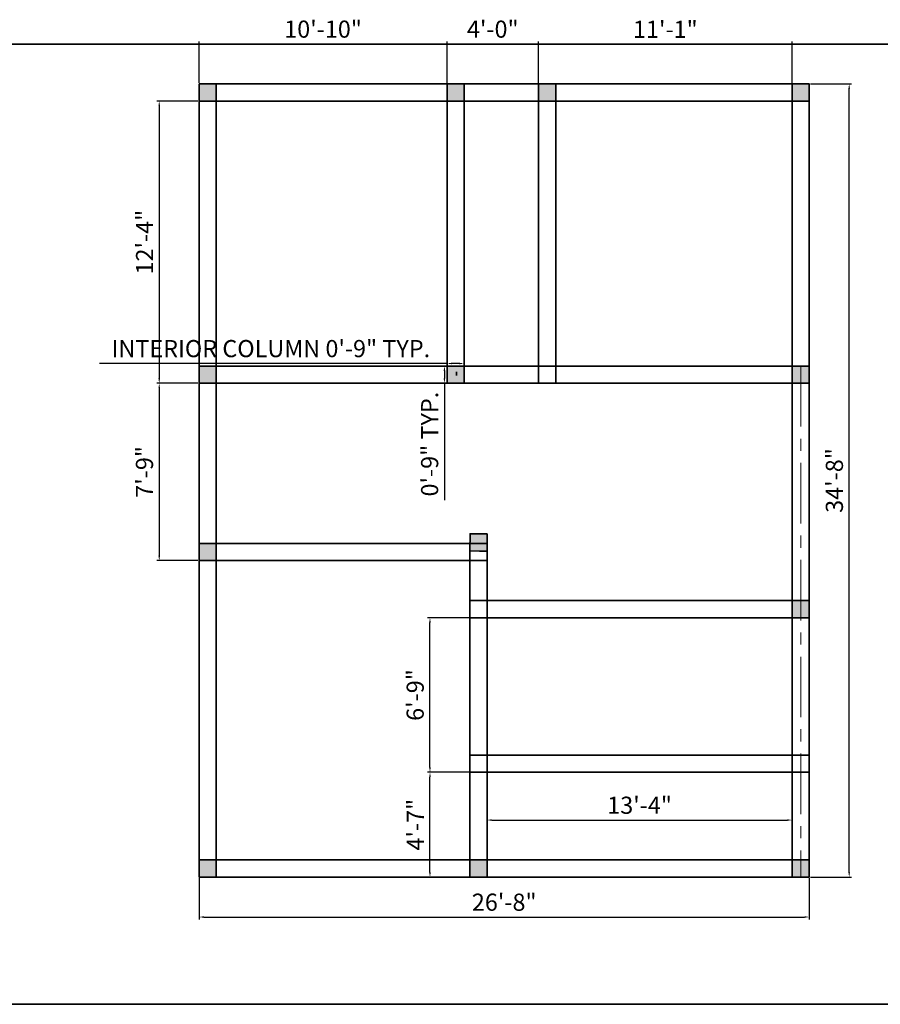
# Model space of a CAD drawing. Units: inches. Extents: x 2289 to 3796, y 1741 to 2286.
# Tile 3 of 4: x 2741 to 3192, y 1742 to 2258. Entities that reach past the tile are written whole.
import ezdxf

# ---------------------------------------------------------------- set-up
doc = ezdxf.new("R2010")
doc.units = ezdxf.units.IN
doc.linetypes.add('CENTER', pattern=[50.8, 31.75, -6.35, 6.35, -6.35])
for name, color, linetype, lineweight in [('A-ANNO-DIMS', 2, 'Continuous', 18), ('A-ANNO-TTLB', 7, 'Continuous', 35), ('S-BEAM', 7, 'Continuous', 35), ('S-COLS', 1, 'Continuous', 35), ('S-GRID', 8, 'CENTER', 18)]:
    doc.layers.add(name, color=color, linetype=linetype, lineweight=lineweight)
doc.styles.get("Standard").update_dxf_attribs({"font": 'arial.ttf'})
doc.dimstyles.new('ISO-25', dxfattribs={"dimtxt": 9, "dimasz": 2.5, "dimexe": 1.25, "dimexo": 0.625, "dimgap": 2, "dimtad": 1, "dimdec": 1, "dimlunit": 4, "dimtxsty": 'Standard', "dimcen": 2.5, "dimadec": 0, "dimazin": 0, "dimtfac": 1, "dimtdec": 1, "dimtmove": 0, "dimatfit": 3, "dimfxl": 1, "dimarcsym": 0})

# ---------------------------------------------------------------- blocks, each defined once
blk = doc.blocks.new('COL-9X9')
h = blk.add_hatch(color=256)
h.dxf.hatch_style = 1
h.paths.add_polyline_path([(0, 9), (0, 0), (9, 0), (9, 9)])
blk.add_lwpolyline([(0, 9), (9, 9), (9, 0), (0, 0)], close=True)
blk = doc.blocks.new('COL-9X9-INT')
h = blk.add_hatch(color=256)
h.dxf.hatch_style = 1
h.paths.add_polyline_path([(9, 0), (9, 9), (0, 9), (0, 0)])
blk.add_lwpolyline([(0, 9), (9, 9), (9, 0), (0, 0)], close=True)
blk = doc.blocks.new('COL-9X9-STAIR')
h = blk.add_hatch(color=256)
h.dxf.hatch_style = 1
h.paths.add_polyline_path([(9, 0), (9, 9), (0, 9), (0, 0)])
blk.add_lwpolyline([(0.01, 9.14), (9.01, 9.14), (9.01, 0.14), (0.01, 0.14)], close=True)
blk = doc.blocks.new('*D25')
at = {"layer": 'A-ANNO-DIMS', "color": 0, "lineweight": -2, "transparency": 16777216}
for p, q in [((2964.67, 2077.74), (2782.42, 2077.74)), ((2964.67, 2077.01), (2964.67, 2078.99)), ((2971.17, 2077.74), (2967.17, 2077.74)), ((2973.67, 2077.01), (2973.67, 2078.99))]:
    blk.add_line(p, q, dxfattribs=at)
at = {"layer": 'A-ANNO-DIMS', "color": 0, "transparency": 16777216}
for points in [[(2967.17, 2078.15), (2967.17, 2077.32), (2964.67, 2077.74)], [(2971.17, 2078.15), (2971.17, 2077.32), (2973.67, 2077.74)]]:
    blk.add_solid(points, dxfattribs=at)
at = {"layer": 'Defpoints', "color": 0, "transparency": 16777216}
for p in [(2964.67, 2077.74), (2964.67, 2076.39), (2973.67, 2076.39)]:
    blk.add_point(p, dxfattribs=at)
at = {"layer": 'A-ANNO-DIMS', "color": 0, "transparency": 16777216, "insert": (2872.29, 2084.39), "char_height": 9, "attachment_point": 5}
blk.add_mtext('INTERIOR COLUMN 0\'-9" TYP.', dxfattribs=at)
blk = doc.blocks.new('*D26')
at = {"layer": 'A-ANNO-DIMS', "color": 0, "lineweight": -2, "transparency": 16777216}
for p, q in [((2964.05, 2076.39), (2962.07, 2076.39)), ((2963.32, 2073.89), (2963.32, 2069.89)), ((2964.05, 2067.39), (2962.07, 2067.39)), ((2963.32, 2067.39), (2963.32, 2006.03))]:
    blk.add_line(p, q, dxfattribs=at)
at = {"layer": 'A-ANNO-DIMS', "color": 0, "transparency": 16777216}
for points in [[(2962.9, 2073.89), (2963.74, 2073.89), (2963.32, 2076.39)], [(2962.9, 2069.89), (2963.74, 2069.89), (2963.32, 2067.39)]]:
    blk.add_solid(points, dxfattribs=at)
at = {"layer": 'Defpoints', "color": 0, "transparency": 16777216}
for p in [(2964.67, 2076.39), (2963.32, 2067.39), (2964.67, 2067.39)]:
    blk.add_point(p, dxfattribs=at)
at = {"layer": 'A-ANNO-DIMS', "color": 0, "transparency": 16777216, "insert": (2956.73, 2035.46), "char_height": 9, "attachment_point": 5, "rotation": 90}
blk.add_mtext('0\'-9" TYP.', dxfattribs=at)
blk = doc.blocks.new('*D54')
at = {"layer": 'A-ANNO-DIMS', "color": 0, "lineweight": -2, "transparency": 16777216}
for p, q in [((2834.67, 1807.76), (2834.67, 1786.21)), ((3154.67, 1807.76), (3154.67, 1786.21)), ((2837.17, 1787.46), (3152.17, 1787.46))]:
    blk.add_line(p, q, dxfattribs=at)
at = {"layer": 'A-ANNO-DIMS', "color": 0, "transparency": 16777216}
for points in [[(2837.17, 1787.88), (2837.17, 1787.04), (2834.67, 1787.46)], [(3152.17, 1787.88), (3152.17, 1787.04), (3154.67, 1787.46)]]:
    blk.add_solid(points, dxfattribs=at)
at = {"layer": 'Defpoints', "color": 0, "transparency": 16777216}
for p in [(2834.67, 1808.39), (3154.67, 1808.39), (3154.67, 1787.46)]:
    blk.add_point(p, dxfattribs=at)
at = {"layer": 'A-ANNO-DIMS', "color": 0, "transparency": 16777216, "insert": (2994.67, 1794.06), "char_height": 9, "attachment_point": 5}
blk.add_mtext('26\'-8"', dxfattribs=at)
blk = doc.blocks.new('*D55')
at = {"layer": 'A-ANNO-DIMS', "color": 0, "lineweight": -2, "transparency": 16777216}
for p, q in [((3155.3, 2224.39), (3176.85, 2224.39)), ((3175.6, 1810.89), (3175.6, 2221.89)), ((3155.3, 1808.39), (3176.85, 1808.39))]:
    blk.add_line(p, q, dxfattribs=at)
at = {"layer": 'A-ANNO-DIMS', "color": 0, "transparency": 16777216}
for points in [[(3175.18, 2221.89), (3176.01, 2221.89), (3175.6, 2224.39)], [(3175.18, 1810.89), (3176.01, 1810.89), (3175.6, 1808.39)]]:
    blk.add_solid(points, dxfattribs=at)
at = {"layer": 'Defpoints', "color": 0, "transparency": 16777216}
for p in [(3154.67, 2224.39), (3175.6, 2224.39), (3154.67, 1808.39)]:
    blk.add_point(p, dxfattribs=at)
at = {"layer": 'A-ANNO-DIMS', "color": 0, "transparency": 16777216, "insert": (3169, 2016.39), "char_height": 9, "attachment_point": 5, "rotation": 90}
blk.add_mtext('34\'-8"', dxfattribs=at)
blk = doc.blocks.new('*D56')
at = {"layer": 'A-ANNO-DIMS', "color": 0, "lineweight": -2, "transparency": 16777216}
for p, q in [((2834.67, 2225.01), (2834.67, 2246.56)), ((2964.67, 2225.01), (2964.67, 2246.56)), ((2837.17, 2245.31), (2962.17, 2245.31))]:
    blk.add_line(p, q, dxfattribs=at)
at = {"layer": 'A-ANNO-DIMS', "color": 0, "transparency": 16777216}
for points in [[(2837.17, 2245.73), (2837.17, 2244.89), (2834.67, 2245.31)], [(2962.17, 2245.73), (2962.17, 2244.89), (2964.67, 2245.31)]]:
    blk.add_solid(points, dxfattribs=at)
at = {"layer": 'Defpoints', "color": 0, "transparency": 16777216}
for p in [(2964.67, 2245.31), (2834.67, 2224.39), (2964.67, 2224.39)]:
    blk.add_point(p, dxfattribs=at)
at = {"layer": 'A-ANNO-DIMS', "color": 0, "transparency": 16777216, "insert": (2899.67, 2251.91), "char_height": 9, "attachment_point": 5}
blk.add_mtext('10\'-10"', dxfattribs=at)
blk = doc.blocks.new('*D57')
at = {"layer": 'A-ANNO-DIMS', "color": 0, "lineweight": -2, "transparency": 16777216}
for p, q in [((2964.67, 2225.01), (2964.67, 2246.56)), ((3012.67, 2225.01), (3012.67, 2246.56)), ((2967.17, 2245.31), (3010.17, 2245.31))]:
    blk.add_line(p, q, dxfattribs=at)
at = {"layer": 'A-ANNO-DIMS', "color": 0, "transparency": 16777216}
for points in [[(2967.17, 2245.73), (2967.17, 2244.89), (2964.67, 2245.31)], [(3010.17, 2245.73), (3010.17, 2244.89), (3012.67, 2245.31)]]:
    blk.add_solid(points, dxfattribs=at)
at = {"layer": 'Defpoints', "color": 0, "transparency": 16777216}
for p in [(3012.67, 2245.31), (2964.67, 2224.39), (3012.67, 2224.39)]:
    blk.add_point(p, dxfattribs=at)
at = {"layer": 'A-ANNO-DIMS', "color": 0, "transparency": 16777216, "insert": (2988.67, 2251.91), "char_height": 9, "attachment_point": 5}
blk.add_mtext('4\'-0"', dxfattribs=at)
blk = doc.blocks.new('*D58')
at = {"layer": 'A-ANNO-DIMS', "color": 0, "lineweight": -2, "transparency": 16777216}
for p, q in [((3012.67, 2225.01), (3012.67, 2246.56)), ((3145.67, 2225.01), (3145.67, 2246.56)), ((3015.17, 2245.31), (3143.17, 2245.31))]:
    blk.add_line(p, q, dxfattribs=at)
at = {"layer": 'A-ANNO-DIMS', "color": 0, "transparency": 16777216}
for points in [[(3015.17, 2245.73), (3015.17, 2244.89), (3012.67, 2245.31)], [(3143.17, 2245.73), (3143.17, 2244.89), (3145.67, 2245.31)]]:
    blk.add_solid(points, dxfattribs=at)
at = {"layer": 'Defpoints', "color": 0, "transparency": 16777216}
for p in [(3145.67, 2245.31), (3012.67, 2224.39), (3145.67, 2224.39)]:
    blk.add_point(p, dxfattribs=at)
at = {"layer": 'A-ANNO-DIMS', "color": 0, "transparency": 16777216, "insert": (3079.17, 2251.83), "char_height": 9, "attachment_point": 5}
blk.add_mtext('11\'-1"', dxfattribs=at)
blk = doc.blocks.new('*D59')
at = {"layer": 'A-ANNO-DIMS', "color": 0, "lineweight": -2, "transparency": 16777216}
for p, q in [((2985.67, 1818.01), (2985.67, 1839.56)), ((2988.17, 1838.31), (3143.17, 1838.31)), ((3145.67, 1818.01), (3145.67, 1839.56))]:
    blk.add_line(p, q, dxfattribs=at)
at = {"layer": 'A-ANNO-DIMS', "color": 0, "transparency": 16777216}
for points in [[(2988.17, 1838.73), (2988.17, 1837.89), (2985.67, 1838.31)], [(3143.17, 1838.73), (3143.17, 1837.89), (3145.67, 1838.31)]]:
    blk.add_solid(points, dxfattribs=at)
at = {"layer": 'Defpoints', "color": 0, "transparency": 16777216}
for p in [(3145.67, 1838.31), (2985.67, 1817.39), (3145.67, 1817.39)]:
    blk.add_point(p, dxfattribs=at)
at = {"layer": 'A-ANNO-DIMS', "color": 0, "transparency": 16777216, "insert": (3065.67, 1844.91), "char_height": 9, "attachment_point": 5}
blk.add_mtext('13\'-4"', dxfattribs=at)
blk = doc.blocks.new('*D60')
at = {"layer": 'A-ANNO-DIMS', "color": 0, "lineweight": -2, "transparency": 16777216}
for p, q in [((2834.05, 2215.39), (2812.5, 2215.39)), ((2813.75, 2212.89), (2813.75, 2069.89)), ((2834.05, 2067.39), (2812.5, 2067.39))]:
    blk.add_line(p, q, dxfattribs=at)
at = {"layer": 'A-ANNO-DIMS', "color": 0, "transparency": 16777216}
for points in [[(2813.33, 2212.89), (2814.16, 2212.89), (2813.75, 2215.39)], [(2813.33, 2069.89), (2814.16, 2069.89), (2813.75, 2067.39)]]:
    blk.add_solid(points, dxfattribs=at)
at = {"layer": 'Defpoints', "color": 0, "transparency": 16777216}
for p in [(2834.67, 2215.39), (2813.75, 2067.39), (2834.67, 2067.39)]:
    blk.add_point(p, dxfattribs=at)
at = {"layer": 'A-ANNO-DIMS', "color": 0, "transparency": 16777216, "insert": (2807.23, 2141.39), "char_height": 9, "attachment_point": 5, "rotation": 90}
blk.add_mtext('12\'-4"', dxfattribs=at)
blk = doc.blocks.new('*D61')
at = {"layer": 'A-ANNO-DIMS', "color": 0, "lineweight": -2, "transparency": 16777216}
for p, q in [((2834.05, 2067.39), (2812.5, 2067.39)), ((2813.75, 2064.89), (2813.75, 1976.89)), ((2834.05, 1974.39), (2812.5, 1974.39))]:
    blk.add_line(p, q, dxfattribs=at)
at = {"layer": 'A-ANNO-DIMS', "color": 0, "transparency": 16777216}
for points in [[(2813.33, 2064.89), (2814.16, 2064.89), (2813.75, 2067.39)], [(2813.33, 1976.89), (2814.16, 1976.89), (2813.75, 1974.39)]]:
    blk.add_solid(points, dxfattribs=at)
at = {"layer": 'Defpoints', "color": 0, "transparency": 16777216}
for p in [(2834.67, 2067.39), (2813.75, 1974.39), (2834.67, 1974.39)]:
    blk.add_point(p, dxfattribs=at)
at = {"layer": 'A-ANNO-DIMS', "color": 0, "transparency": 16777216, "insert": (2807.15, 2020.89), "char_height": 9, "attachment_point": 5, "rotation": 90}
blk.add_mtext('7\'-9"', dxfattribs=at)
blk = doc.blocks.new('*D62')
at = {"layer": 'A-ANNO-DIMS', "color": 0, "lineweight": -2, "transparency": 16777216}
for p, q in [((2976.05, 1863.39), (2954.5, 1863.39)), ((2955.75, 1810.89), (2955.75, 1860.89)), ((2976.05, 1808.39), (2954.5, 1808.39))]:
    blk.add_line(p, q, dxfattribs=at)
at = {"layer": 'A-ANNO-DIMS', "color": 0, "transparency": 16777216}
for points in [[(2955.33, 1860.89), (2956.16, 1860.89), (2955.75, 1863.39)], [(2955.33, 1810.89), (2956.16, 1810.89), (2955.75, 1808.39)]]:
    blk.add_solid(points, dxfattribs=at)
at = {"layer": 'Defpoints', "color": 0, "transparency": 16777216}
for p in [(2955.75, 1863.39), (2976.67, 1863.39), (2976.67, 1808.39)]:
    blk.add_point(p, dxfattribs=at)
at = {"layer": 'A-ANNO-DIMS', "color": 0, "transparency": 16777216, "insert": (2949.25, 1835.89), "char_height": 9, "attachment_point": 5, "rotation": 90}
blk.add_mtext('4\'-7"', dxfattribs=at)
blk = doc.blocks.new('*D63')
at = {"layer": 'A-ANNO-DIMS', "color": 0, "lineweight": -2, "transparency": 16777216}
for p, q in [((2976.05, 1944.39), (2954.5, 1944.39)), ((2955.75, 1865.89), (2955.75, 1941.89)), ((2976.05, 1863.39), (2954.5, 1863.39))]:
    blk.add_line(p, q, dxfattribs=at)
at = {"layer": 'A-ANNO-DIMS', "color": 0, "transparency": 16777216}
for points in [[(2955.33, 1941.89), (2956.16, 1941.89), (2955.75, 1944.39)], [(2955.33, 1865.89), (2956.16, 1865.89), (2955.75, 1863.39)]]:
    blk.add_solid(points, dxfattribs=at)
at = {"layer": 'Defpoints', "color": 0, "transparency": 16777216}
for p in [(2955.75, 1944.39), (2976.67, 1944.39), (2976.67, 1863.39)]:
    blk.add_point(p, dxfattribs=at)
at = {"layer": 'A-ANNO-DIMS', "color": 0, "transparency": 16777216, "insert": (2949.15, 1903.89), "char_height": 9, "attachment_point": 5, "rotation": 90}
blk.add_mtext('6\'-9"', dxfattribs=at)

msp = doc.modelspace()

# ---------------------------------------------------------------- linework, layer by layer
at = {"layer": 'A-ANNO-TTLB'}
msp.add_lwpolyline([(2318.16, 2245.19), (3750.19, 2245.19), (3750.19, 1741.69), (2318.16, 1741.69)], close=True, dxfattribs=at)
at = {"layer": 'S-BEAM'}
for p, q in [((2834.67, 2224.39), (3154.67, 2224.39)), ((2834.67, 2224.39), (2834.67, 1808.39)), ((2964.67, 2224.39), (2964.67, 2071.39)), ((2973.67, 2224.39), (2973.67, 2071.39)), ((3012.67, 2224.39), (3012.67, 2067.39)), ((3021.67, 2224.39), (3021.67, 2071.39)), ((3154.67, 2224.39), (3154.67, 1808.39)), ((2843.67, 2215.39), (2969.67, 2215.39)), ((2843.67, 2215.39), (3154.67, 2215.39)), ((2843.67, 2215.39), (2843.67, 2071.39)), ((2973.67, 2215.39), (3021.67, 2215.39)), ((3145.67, 2215.39), (3145.67, 2067.39)), ((3021.67, 2127.39), (3021.67, 2067.39)), ((2834.67, 2076.39), (3154.67, 2076.39)), ((3145.67, 2076.39), (3145.67, 1808.39)), ((2969.67, 2073.39), (2969.67, 2071.39)), ((2973.67, 2073.39), (2973.67, 2067.39)), ((2834.67, 2067.39), (3154.67, 2067.39)), ((2843.67, 2067.39), (2843.67, 1983.39)), ((3021.67, 2067.39), (3027.67, 2067.39)), ((3063.67, 2067.39), (3154.67, 2067.39)), ((2834.67, 1983.39), (2985.67, 1983.39)), ((2976.67, 1983.39), (2976.67, 1808.39)), ((2979.67, 1983.39), (2981.67, 1983.39)), ((2981.67, 1983.39), (2985.67, 1983.39)), ((2985.67, 1983.39), (2985.67, 1817.39)), ((2843.67, 1979.39), (2843.67, 1817.39)), ((2981.67, 1979.39), (2985.67, 1979.39)), ((2834.67, 1974.39), (2985.67, 1974.39)), ((2976.67, 1953.39), (3154.67, 1953.39)), ((3145.67, 1953.39), (3145.67, 1817.39)), ((2976.67, 1944.39), (3154.67, 1944.39)), ((2976.67, 1872.39), (3154.67, 1872.39)), ((2985.67, 1868.39), (2985.67, 1808.39)), ((3145.67, 1868.39), (3145.67, 1808.39)), ((2976.67, 1863.39), (3154.67, 1863.39)), ((2834.67, 1817.39), (3145.67, 1817.39)), ((2976.67, 1817.39), (2976.67, 1808.39)), ((3145.67, 1817.39), (3154.67, 1817.39)), ((2834.67, 1808.39), (3154.67, 1808.39))]:
    msp.add_line(p, q, dxfattribs=at)
at = {"layer": 'S-GRID'}
msp.add_line((3150.17, 2076.39), (3150.17, 1808.39), dxfattribs=at)

# ---------------------------------------------------------------- block references
at = {"layer": 'S-COLS'}
for p in [(2834.67, 2215.39), (2964.67, 2215.39), (3012.67, 2215.39), (3145.67, 2215.39), (2834.67, 2067.39), (3145.67, 2067.39), (2834.67, 1974.39), (3145.67, 1944.39), (2834.67, 1808.39), (2976.67, 1808.39), (3145.67, 1808.39)]:
    msp.add_blockref('COL-9X9', p, dxfattribs=at)
for name, p, rotation in [('COL-9X9-INT', (2973.67, 2076.39), 180), ('COL-9X9-STAIR', (2976.66, 1988.51), 269.119134070298)]:
    msp.add_blockref(name, p, dxfattribs=dict(at, rotation=rotation))

# ---------------------------------------------------------------- dimensions: what is measured, and where the dimension line sits
at = {"layer": 'A-ANNO-DIMS'}
for base, p1, p2, picture, middle in [((2964.67, 2245.31), (2834.67, 2224.39), (2964.67, 2224.39), '*D56', (2899.67, 2251.91)), ((3012.67, 2245.31), (2964.67, 2224.39), (3012.67, 2224.39), '*D57', (2988.67, 2251.91)), ((3145.67, 2245.31), (3012.67, 2224.39), (3145.67, 2224.39), '*D58', (3079.17, 2251.83)), ((3154.67, 1787.46), (2834.67, 1808.39), (3154.67, 1808.39), '*D54', (2994.67, 1794.06))]:
    dim = msp.add_linear_dim(base=base, p1=p1, p2=p2, dimstyle='ISO-25', override={"dimdec": 1, "dimlfac": 1, "dimrnd": 0, "dimzin": 1, "dimdsep": 46, "dimlunit": 4, "dimfrac": 2}, dxfattribs=at)
    dim.commit()
    dim.dimension.update_dxf_attribs({"geometry": picture, "text_midpoint": middle})
for base, p1, p2, angle, picture, middle in [((3175.6, 2224.39), (3154.67, 1808.39), (3154.67, 2224.39), 90, '*D55', (3169, 2016.39)), ((2813.75, 2067.39), (2834.67, 2215.39), (2834.67, 2067.39), 90, '*D60', (2807.23, 2141.39)), ((2813.75, 1974.39), (2834.67, 2067.39), (2834.67, 1974.39), 90, '*D61', (2807.15, 2020.89)), ((2955.75, 1944.39), (2976.67, 1863.39), (2976.67, 1944.39), 90, '*D63', (2949.15, 1903.89)), ((2955.75, 1863.39), (2976.67, 1808.39), (2976.67, 1863.39), 90, '*D62', (2949.25, 1835.89)), ((3145.67, 1838.31), (2985.67, 1817.39), (3145.67, 1817.39), 0, '*D59', (3065.67, 1844.91))]:
    dim = msp.add_linear_dim(base=base, p1=p1, p2=p2, angle=angle, dimstyle='ISO-25', override={"dimdec": 1, "dimlfac": 1, "dimrnd": 0, "dimzin": 1, "dimdsep": 46, "dimlunit": 4, "dimfrac": 2}, dxfattribs=at)
    dim.commit()
    dim.dimension.update_dxf_attribs({"geometry": picture, "text_midpoint": middle})
for base, p1, p2, angle, text, picture, middle in [((2964.67, 2077.74), (2973.67, 2076.39), (2964.67, 2076.39), 180, 'INTERIOR COLUMN <> TYP.', '*D25', (2872.29, 2084.39)), ((2963.32, 2067.39), (2964.67, 2076.39), (2964.67, 2067.39), 270, '<> TYP.', '*D26', (2956.73, 2035.46))]:
    dim = msp.add_linear_dim(base=base, p1=p1, p2=p2, angle=angle, text=text, dimstyle='ISO-25', override={"dimdec": 1, "dimlfac": 1, "dimrnd": 0, "dimzin": 1, "dimdsep": 46, "dimlunit": 4, "dimfrac": 2}, dxfattribs=at)
    dim.commit()
    dim.dimension.update_dxf_attribs({"geometry": picture, "text_midpoint": middle})

doc.saveas('drawing.dxf')
